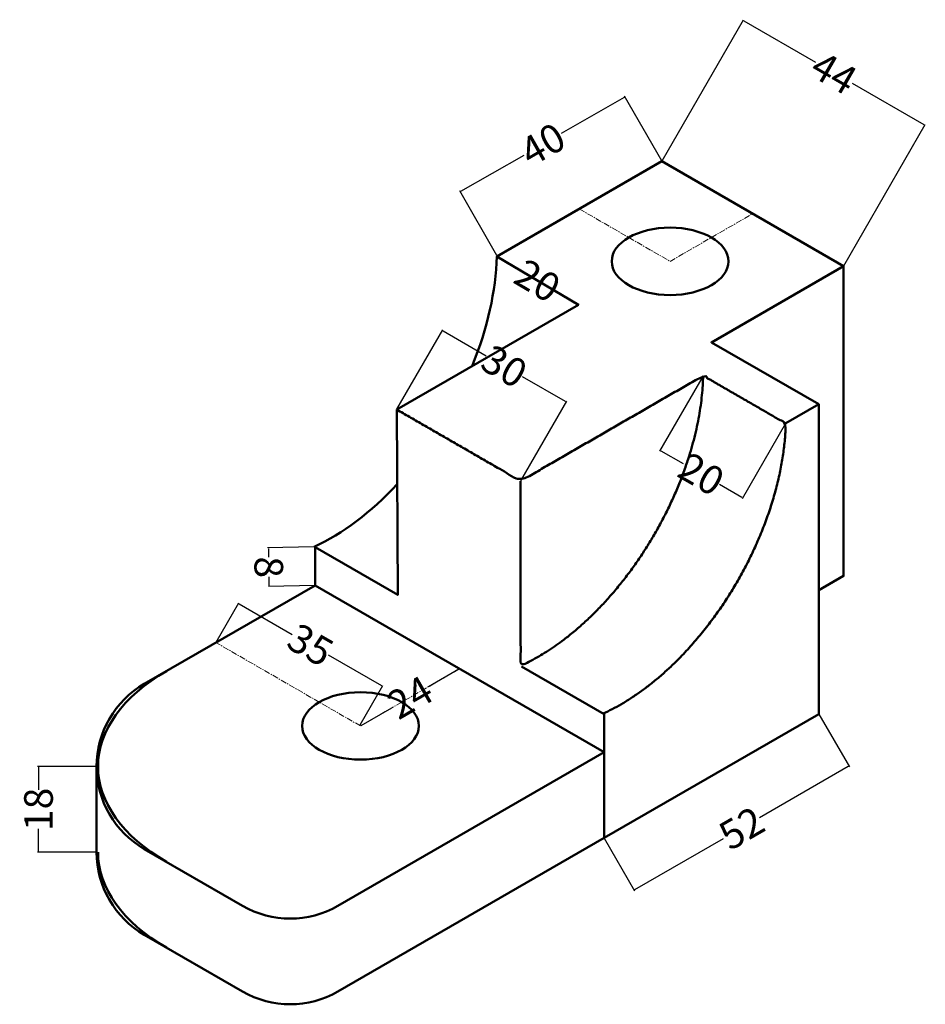
# Model space of a CAD drawing. Units: millimetres. Extents: x -105 to 85, y 93 to 299.
import ezdxf

# ---------------------------------------------------------------- set-up
doc = ezdxf.new("R2010")
doc.units = ezdxf.units.MM
doc.header["$MEASUREMENT"] = 0
doc.linetypes.add('CENTER', pattern=[2, 1.25, -0.25, 0.25, -0.25])
for name, color, linetype, lineweight in [('M-CNTR', 4, 'CENTER', 18), ('M-DIMS', 2, 'Continuous', 25), ('M-OUTL', 7, 'Continuous', 50)]:
    doc.layers.add(name, color=color, linetype=linetype, lineweight=lineweight)
doc.styles.get("Standard").update_dxf_attribs({"font": 'arial.ttf'})
doc.dimstyles.get("Standard").update_dxf_attribs({"dimtxt": 6, "dimasz": 0.18, "dimexe": 0.18, "dimexo": 0.0625, "dimgap": 0.09, "dimtad": 0, "dimtoh": 1, "dimdec": 0, "dimzin": 0, "dimdsep": 46, "dimtxsty": 'Standard', "dimcen": 0.09, "dimadec": 0, "dimazin": 0, "dimtfac": 1, "dimtdec": 0, "dimtofl": 0, "dimtmove": 0, "dimatfit": 3, "dimfxl": 1, "dimtolj": 1, "dimtzin": 0, "dimarcsym": 0})

# ---------------------------------------------------------------- blocks, each defined once
blk = doc.blocks.new('*D1')
at = {"layer": 'Defpoints', "color": 0, "transparency": 16777216}
for p in [(-12.61, 163.21), (-12.61, 163.21), (-33.4, 151.21)]:
    blk.add_point(p, dxfattribs=at)
at = {"layer": 'M-DIMS', "color": 0, "lineweight": -2, "transparency": 16777216}
for p, q in [((-12.64, 163.26), (-12.7, 163.36)), ((-12.77, 163.12), (-19.17, 159.42)), ((-33.24, 151.3), (-26.84, 155)), ((-33.43, 151.26), (-33.49, 151.36))]:
    blk.add_line(p, q, dxfattribs=at)
at = {"layer": 'M-DIMS', "color": 0, "transparency": 16777216}
for points in [[(-12.78, 163.14), (-12.75, 163.09), (-12.61, 163.21)], [(-33.26, 151.32), (-33.23, 151.27), (-33.4, 151.21)]]:
    blk.add_solid(points, dxfattribs=at)
at = {"layer": 'M-DIMS', "color": 0, "transparency": 16777216, "insert": (-23, 157.21), "char_height": 6, "attachment_point": 5, "rotation": 30}
blk.add_mtext('\\A1;24', dxfattribs=at)
blk = doc.blocks.new('*D2')
at = {"layer": 'Defpoints', "color": 0, "transparency": 16777216}
for p in [(-59.01, 176.89), (-63.71, 168.71), (-33.49, 151.36)]:
    blk.add_point(p, dxfattribs=at)
at = {"layer": 'M-DIMS', "color": 0, "lineweight": -2, "transparency": 16777216}
for p, q in [((-63.68, 168.76), (-58.92, 177.05)), ((-58.85, 176.8), (-47.72, 170.42)), ((-28.95, 159.64), (-40.08, 166.03)), ((-33.46, 151.42), (-28.7, 159.71))]:
    blk.add_line(p, q, dxfattribs=at)
at = {"layer": 'M-DIMS', "color": 0, "transparency": 16777216}
for points in [[(-58.84, 176.83), (-58.87, 176.78), (-59.01, 176.89)], [(-28.93, 159.66), (-28.96, 159.61), (-28.79, 159.55)]]:
    blk.add_solid(points, dxfattribs=at)
at = {"layer": 'M-DIMS', "color": 0, "transparency": 16777216, "insert": (-43.9, 168.22), "char_height": 6, "attachment_point": 5, "rotation": 330.148}
blk.add_mtext('\\A1;35', dxfattribs=at)
blk = doc.blocks.new('*D3')
at = {"layer": 'Defpoints', "color": 0, "transparency": 16777216}
for p in [(-88.74, 142.71), (-100.94, 124.71), (-88.74, 124.71)]:
    blk.add_point(p, dxfattribs=at)
at = {"layer": 'M-DIMS', "color": 0, "lineweight": -2, "transparency": 16777216}
for p, q in [((-88.8, 142.71), (-101.12, 142.71)), ((-100.94, 142.53), (-100.94, 137.82)), ((-100.94, 124.89), (-100.94, 129.6)), ((-88.8, 124.71), (-101.12, 124.71))]:
    blk.add_line(p, q, dxfattribs=at)
at = {"layer": 'M-DIMS', "color": 0, "transparency": 16777216}
for points in [[(-100.97, 142.53), (-100.91, 142.53), (-100.94, 142.71)], [(-100.97, 124.89), (-100.91, 124.89), (-100.94, 124.71)]]:
    blk.add_solid(points, dxfattribs=at)
at = {"layer": 'M-DIMS', "color": 0, "transparency": 16777216, "insert": (-100.94, 133.71), "char_height": 6, "attachment_point": 5, "rotation": 90}
blk.add_mtext('\\A1;18', dxfattribs=at)
blk = doc.blocks.new('*D4')
at = {"layer": 'Defpoints', "color": 0, "transparency": 16777216}
for p in [(-43.12, 188.82), (-52.54, 180.48), (-42.92, 180.71)]:
    blk.add_point(p, dxfattribs=at)
at = {"layer": 'M-DIMS', "color": 0, "lineweight": -2, "transparency": 16777216}
for p, q in [((-43.18, 188.82), (-52.91, 188.59)), ((-52.72, 188.41), (-52.68, 186.6)), ((-52.54, 180.66), (-52.58, 182.47)), ((-42.99, 180.71), (-52.72, 180.47))]:
    blk.add_line(p, q, dxfattribs=at)
at = {"layer": 'M-DIMS', "color": 0, "transparency": 16777216}
for points in [[(-52.69, 188.41), (-52.75, 188.41), (-52.73, 188.59)], [(-52.51, 180.66), (-52.57, 180.66), (-52.54, 180.48)]]:
    blk.add_solid(points, dxfattribs=at)
at = {"layer": 'M-DIMS', "color": 0, "transparency": 16777216, "insert": (-52.63, 184.54), "char_height": 6, "attachment_point": 5, "rotation": 271.3676}
blk.add_mtext('\\A1;8', dxfattribs=at)
blk = doc.blocks.new('*D5')
at = {"layer": 'Defpoints', "color": 0, "transparency": 16777216}
for p in [(-4.83, 249.7), (12.31, 239.6), (12.31, 239.6)]:
    blk.add_point(p, dxfattribs=at)
at = {"layer": 'M-DIMS', "color": 0, "lineweight": -2, "transparency": 16777216}
for p, q in [((-4.8, 249.76), (-4.74, 249.86)), ((-4.67, 249.61), (-0.07, 246.9)), ((12.15, 239.69), (7.56, 242.4)), ((12.34, 239.65), (12.4, 239.75))]:
    blk.add_line(p, q, dxfattribs=at)
at = {"layer": 'M-DIMS', "color": 0, "transparency": 16777216}
for points in [[(-4.66, 249.64), (-4.69, 249.59), (-4.83, 249.7)], [(12.17, 239.71), (12.14, 239.66), (12.31, 239.6)]]:
    blk.add_solid(points, dxfattribs=at)
at = {"layer": 'M-DIMS', "color": 0, "transparency": 16777216, "insert": (3.74, 244.65), "char_height": 6, "attachment_point": 5, "rotation": 329.4735}
blk.add_mtext('\\A1;20', dxfattribs=at)
blk = doc.blocks.new('*D6')
at = {"layer": 'Defpoints', "color": 0, "transparency": 16777216}
for p in [(9.76, 219.18), (-25.8, 217.6), (0.19, 202.6)]:
    blk.add_point(p, dxfattribs=at)
at = {"layer": 'M-DIMS', "color": 0, "lineweight": -2, "transparency": 16777216}
for p, q in [((-25.76, 217.65), (-16.13, 234.33)), ((-16.07, 234.09), (-7.02, 228.86)), ((9.6, 219.27), (0.56, 224.49)), ((0.22, 202.65), (9.85, 219.33))]:
    blk.add_line(p, q, dxfattribs=at)
at = {"layer": 'M-DIMS', "color": 0, "transparency": 16777216}
for points in [[(-16.05, 234.11), (-16.08, 234.06), (-16.22, 234.18)], [(9.62, 219.29), (9.59, 219.24), (9.76, 219.18)]]:
    blk.add_solid(points, dxfattribs=at)
at = {"layer": 'M-DIMS', "color": 0, "transparency": 16777216, "insert": (-3.23, 226.68), "char_height": 6, "attachment_point": 5, "rotation": 330}
blk.add_mtext('\\A1;30', dxfattribs=at)
blk = doc.blocks.new('*D7')
at = {"layer": 'Defpoints', "color": 0, "transparency": 16777216}
for p in [(38.47, 224.7), (55.79, 214.7), (46.76, 199.05)]:
    blk.add_point(p, dxfattribs=at)
at = {"layer": 'M-DIMS', "color": 0, "lineweight": -2, "transparency": 16777216}
for p, q in [((38.44, 224.65), (29.35, 208.89)), ((55.76, 214.65), (46.67, 198.89)), ((29.59, 208.96), (34.26, 206.26)), ((46.6, 199.14), (41.93, 201.84))]:
    blk.add_line(p, q, dxfattribs=at)
at = {"layer": 'M-DIMS', "color": 0, "transparency": 16777216}
for points in [[(29.61, 208.99), (29.58, 208.93), (29.44, 209.05)], [(46.62, 199.17), (46.59, 199.11), (46.76, 199.05)]]:
    blk.add_solid(points, dxfattribs=at)
at = {"layer": 'M-DIMS', "color": 0, "transparency": 16777216, "insert": (38.1, 204.05), "char_height": 6, "attachment_point": 5, "rotation": 330}
blk.add_mtext('\\A1;20', dxfattribs=at)
blk = doc.blocks.new('*D8')
at = {"layer": 'Defpoints', "color": 0, "transparency": 16777216}
for p in [(22.08, 283.17), (29.81, 269.7), (-4.74, 249.86)]:
    blk.add_point(p, dxfattribs=at)
at = {"layer": 'M-DIMS', "color": 0, "lineweight": -2, "transparency": 16777216}
for p, q in [((21.92, 283.08), (8.7, 275.49)), ((29.78, 269.76), (21.99, 283.33)), ((-12.32, 263.42), (0.9, 271.01)), ((-4.77, 249.91), (-12.56, 263.48))]:
    blk.add_line(p, q, dxfattribs=at)
at = {"layer": 'M-DIMS', "color": 0, "transparency": 16777216}
for points in [[(21.91, 283.11), (21.94, 283.06), (22.08, 283.17)], [(-12.33, 263.44), (-12.3, 263.39), (-12.47, 263.33)]]:
    blk.add_solid(points, dxfattribs=at)
at = {"layer": 'M-DIMS', "color": 0, "transparency": 16777216, "insert": (4.8, 273.25), "char_height": 6, "attachment_point": 5, "rotation": 29.8726}
blk.add_mtext('\\A1;40', dxfattribs=at)
blk = doc.blocks.new('*D9')
at = {"layer": 'Defpoints', "color": 0, "transparency": 16777216}
for p in [(84.98, 277.25), (29.81, 269.7), (67.92, 247.7)]:
    blk.add_point(p, dxfattribs=at)
at = {"layer": 'M-DIMS', "color": 0, "lineweight": -2, "transparency": 16777216}
for p, q in [((29.84, 269.76), (46.96, 299.4)), ((47.03, 299.16), (62.03, 290.5)), ((84.82, 277.34), (69.82, 286)), ((67.95, 247.76), (85.07, 277.4))]:
    blk.add_line(p, q, dxfattribs=at)
at = {"layer": 'M-DIMS', "color": 0, "transparency": 16777216}
for points in [[(47.04, 299.18), (47.01, 299.13), (46.87, 299.25)], [(84.84, 277.36), (84.81, 277.31), (84.98, 277.25)]]:
    blk.add_solid(points, dxfattribs=at)
at = {"layer": 'M-DIMS', "color": 0, "transparency": 16777216, "insert": (65.92, 288.25), "char_height": 6, "attachment_point": 5, "rotation": 330}
blk.add_mtext('\\A1;44', dxfattribs=at)
blk = doc.blocks.new('*D10')
at = {"layer": 'Defpoints', "color": 0, "transparency": 16777216}
for p in [(62.73, 153.71), (69.05, 142.77), (17.7, 127.71)]:
    blk.add_point(p, dxfattribs=at)
at = {"layer": 'M-DIMS', "color": 0, "lineweight": -2, "transparency": 16777216}
for p, q in [((62.76, 153.65), (69.14, 142.61)), ((68.89, 142.68), (50.3, 131.95)), ((17.73, 127.65), (24.1, 116.61)), ((24.17, 116.86), (42.76, 127.59))]:
    blk.add_line(p, q, dxfattribs=at)
at = {"layer": 'M-DIMS', "color": 0, "transparency": 16777216}
for points in [[(68.88, 142.71), (68.91, 142.65), (69.05, 142.77)], [(24.16, 116.89), (24.19, 116.83), (24.01, 116.77)]]:
    blk.add_solid(points, dxfattribs=at)
at = {"layer": 'M-DIMS', "color": 0, "transparency": 16777216, "insert": (46.53, 129.77), "char_height": 6, "attachment_point": 5, "rotation": 30}
blk.add_mtext('\\A1;52', dxfattribs=at)

msp = doc.modelspace()

# ---------------------------------------------------------------- linework, layer by layer
at = {"layer": 'M-CNTR'}
for points in [[(12.49, 259.7), (31.54, 248.7), (48.87, 258.7)], [(-12.61, 163.21), (-33.4, 151.21), (-63.71, 168.71)]]:
    msp.add_lwpolyline(points, dxfattribs=at)
at = {"layer": 'M-OUTL'}
msp.add_line((-25.6, 198.71), (-25.6, 198.71), dxfattribs=at)
for points in [[(-42.92, 180.71), (17.7, 145.71), (-38.12, 113.48, -0.267949), (-58.12, 113.48), (-78.74, 125.39, -0.57735), (-78.74, 160.03), (-42.92, 180.71), (-42.92, 188.71), (-25.6, 178.71), (-25.8, 217.6), (12.31, 239.6), (-4.83, 249.7), (29.81, 269.7), (67.92, 247.7), (67.92, 182.7), (62.73, 179.71)], [(17.7, 127.71), (-38.12, 95.48, -0.267949), (-58.12, 95.48), (-78.74, 107.39, -0.267949), (-88.74, 124.71), (-88.74, 142.71)]]:
    msp.add_lwpolyline(points, format="xyb", dxfattribs=at)
for points in [[(67.92, 247.7), (40.21, 231.7), (62.73, 218.71), (62.73, 153.71), (17.7, 127.71), (17.7, 145.71), (17.7, 153.71)], [(55.79, 214.7), (55.8, 214.71), (62.73, 218.71)], [(0.38, 163.71), (17.7, 153.71), (17.7, 153.91)]]:
    msp.add_lwpolyline(points, dxfattribs=at)
for centre in [(31.54, 248.7), (-33.4, 151.21)]:
    msp.add_ellipse(centre, major_axis=(-12.25, 0), ratio=0.57735, dxfattribs=at)
for centre, major_axis, start_param, end_param in [((-39.46, 230.71), (-24.49, -42.43), 8.086673, 8.614384), ((-39.46, 230.71), (-24.49, -42.43), 6.962796, 7.476462), ((-39.46, 142.71), (48.99, 0), 2.356192, 3.141593), ((-39.46, 142.71), (48.99, 0), 3.141593, 3.926993), ((-39.46, 124.71), (48.99, 0), 3.141593, 3.926993)]:
    msp.add_ellipse(centre, major_axis=major_axis, ratio=0.57735, start_param=start_param, end_param=end_param, dxfattribs=at)
for points, weights, knots in [([(17.51, 153.82), (32.6, 160.68), (44.01, 178.82), (55.41, 196.97), (55.79, 214.7), (47.13, 219.7), (38.47, 224.7), (19.33, 213.65), (0.19, 202.6), (-12.81, 210.1), (-25.8, 217.6)], [1, 0.915962174263, 1, 0.915962174263, 1, 1, 1, 1, 1, 1, 1], [0, 0, 0, 0.825794, 0.825794, 1.651588, 1.651588, 2.651588, 2.651588, 3.651588, 3.651588, 4.651588, 4.651588, 4.651588]), ([(0.19, 202.6), (0.19, 183.21), (0.19, 163.82), (15.28, 170.68), (26.68, 188.82), (38.09, 206.97), (38.47, 224.7)], [1, 1, 1, 0.915962174263, 1, 0.915962174263, 1], [0, 0, 0, 1, 1, 1.825794, 1.825794, 2.651588, 2.651588, 2.651588])]:
    msp.add_rational_spline(points, weights, degree=2, knots=knots, dxfattribs=at)

# ---------------------------------------------------------------- dimensions: what is measured, and where the dimension line sits
at = {"layer": 'M-DIMS'}
for p1, p2, distance, picture, middle in [((29.81, 269.7), (67.92, 247.7), 34.12, '*D9', (65.92, 288.25)), ((-4.74, 249.86), (29.81, 269.7), 15.53, '*D8', (4.8, 273.25)), ((-4.83, 249.7), (12.31, 239.6), 0, '*D5', (3.74, 244.65)), ((-25.8, 217.6), (0.19, 202.6), 19.14, '*D6', (-3.23, 226.68)), ((38.47, 224.7), (55.79, 214.7), -18.07, '*D7', (38.1, 204.05)), ((-43.12, 188.82), (-42.92, 180.71), -9.62, '*D4', (-52.63, 184.54)), ((-33.49, 151.36), (-63.71, 168.71), -9.44, '*D2', (-43.9, 168.22)), ((-33.4, 151.21), (-12.61, 163.21), 0, '*D1', (-23, 157.21)), ((17.7, 127.71), (62.73, 153.71), -12.63, '*D10', (46.53, 129.77)), ((-88.74, 142.71), (-88.74, 124.71), -12.2, '*D3', (-100.94, 133.71))]:
    dim = msp.add_aligned_dim(p1=p1, p2=p2, distance=distance, dimstyle='Standard', override={"dimclrd": 0, "dimclre": 0, "dimclrt": 0}, dxfattribs=at)
    dim.commit()
    dim.dimension.update_dxf_attribs({"geometry": picture, "text_midpoint": middle})

doc.saveas('drawing.dxf')
